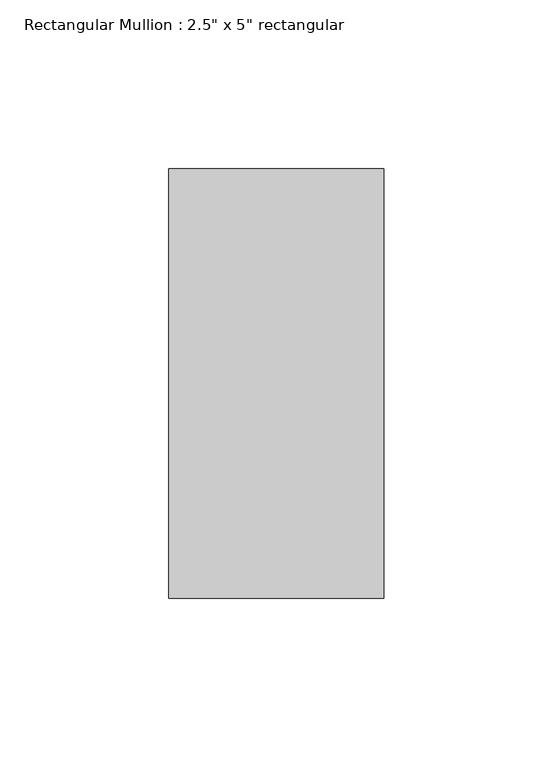
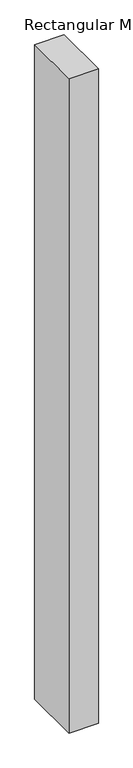
"""IFC4 building model written with IfcOpenShell, lengths in millimetres: member geometry."""

from ifc_helpers import new_model, si_unit, frame, origin, place, context, project, spatial, polyline, outline, extrude, source, transform, mapped, element, save


def member_bc64557a(model_context):
    return source(origin(), model_context, "Body", "SweptSolid", [
        extrude(outline(polyline([(31.75, 63.5), (31.75, -63.5), (-31.75, -63.5), (-31.75, 63.5), (31.75, 63.5)])), frame((0.0, 0.0, -1486.8504732), z_axis=(0.0, 0.0, 1.0), x_axis=(1.0, 0.0, 0.0)), (0.0, 0.0, 1.0), 1486.8504732),
    ])


if __name__ == "__main__":
    model = new_model("IFC4")
    model_context = context("Model", 3, world=origin())
    ifc_project = project(units=[si_unit("LENGTHUNIT", "METRE", prefix="MILLI")], contexts=[model_context])
    site = spatial("IfcSite", under=ifc_project)
    building = spatial("IfcBuilding", under=site)
    placement = place(None, origin())
    member_shape = member_bc64557a(model_context)
    element("IfcMember", 1, ObjectType="Rectangular Mullion : 2.5\" x 5\" rectangular", at=placement, inside=building, context=model_context, shape_type="MappedRepresentation", body=[
        mapped(member_shape, transform((0.0, 0.0, 0.0), x_axis=(1.0, 0.0, 0.0), y_axis=(0.0, 1.0, 0.0), z_axis=(0.0, 0.0, 1.0))),
    ])
    save(model, "model.ifc")

# Revit data of these elements
# Type "Rectangular Mullion : 2.5\" x 5\" rectangular"
#   built-in parameter 1007304 = 0.416667 (stored number, unit not read)
#   built-in parameter 1007301 = 0.104167 (stored number, unit not read)
#   built-in parameter 1007300 = 0.104167 (stored number, unit not read)
# Element 1 (IfcMember, "Rectangular Mullion : 2.5\" x 5\" rectangular")
#   Materials on its faces: "Aluminum"
# Materials
#   "Aluminum": class "Metal", colour RGB 247 247 247, transparency 0, Description = "Aluminum 6061", Cost = 0
